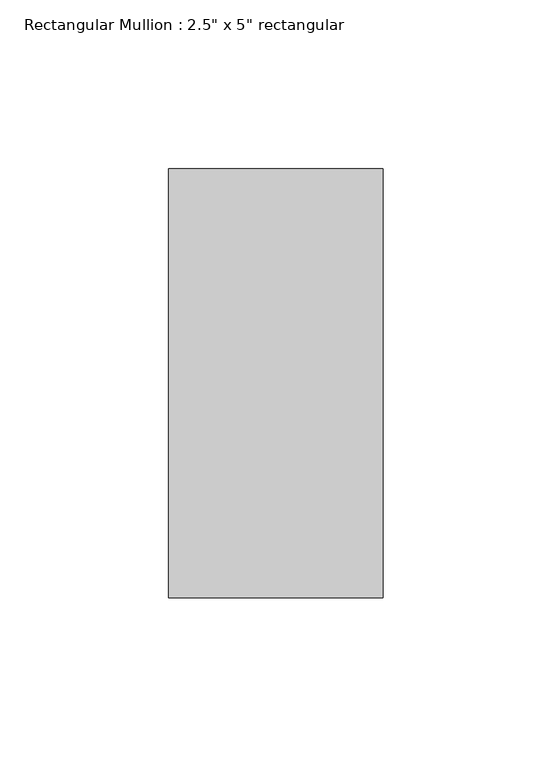
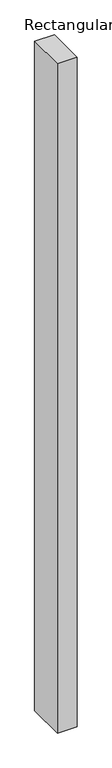
"""IFC4 building model written with IfcOpenShell, lengths in millimetres: member geometry."""

from ifc_helpers import new_model, si_unit, frame, origin, place, context, project, spatial, polyline, outline, extrude, source, transform, mapped, element, save


def member_222163d1(model_context):
    return source(origin(), model_context, "Body", "SweptSolid", [
        extrude(outline(polyline([(31.75, 63.5), (31.75, -63.5), (-31.75, -63.5), (-31.75, 63.5), (31.75, 63.5)])), frame((0.0, 0.0, -2286.0), z_axis=(0.0, 0.0, 1.0), x_axis=(1.0, 0.0, 0.0)), (0.0, 0.0, 1.0), 2286.0),
    ])


if __name__ == "__main__":
    model = new_model("IFC4")
    model_context = context("Model", 3, world=origin())
    ifc_project = project(units=[si_unit("LENGTHUNIT", "METRE", prefix="MILLI")], contexts=[model_context])
    site = spatial("IfcSite", under=ifc_project)
    building = spatial("IfcBuilding", under=site)
    placement = place(None, origin())
    member_shape = member_222163d1(model_context)
    element("IfcMember", 1, ObjectType="Rectangular Mullion : 2.5\" x 5\" rectangular", at=placement, inside=building, context=model_context, shape_type="MappedRepresentation", body=[
        mapped(member_shape, transform((0.0, 0.0, 0.0), x_axis=(1.0, 0.0, 0.0), y_axis=(0.0, 1.0, 0.0), z_axis=(0.0, 0.0, 1.0))),
    ])
    save(model, "model.ifc")

# Revit data of these elements
# Type "Rectangular Mullion : 2.5\" x 5\" rectangular"
#   built-in parameter 1007304 = 0.416667 (stored number, unit not read)
#   built-in parameter 1007301 = 0.104167 (stored number, unit not read)
#   built-in parameter 1007300 = 0.104167 (stored number, unit not read)
# Element 1 (IfcMember, "Rectangular Mullion : 2.5\" x 5\" rectangular")
#   Materials on its faces: "Aluminum"
# Materials
#   "Aluminum": class "Metal", colour RGB 247 247 247, transparency 0, Description = "Aluminum 6061", Cost = 0
